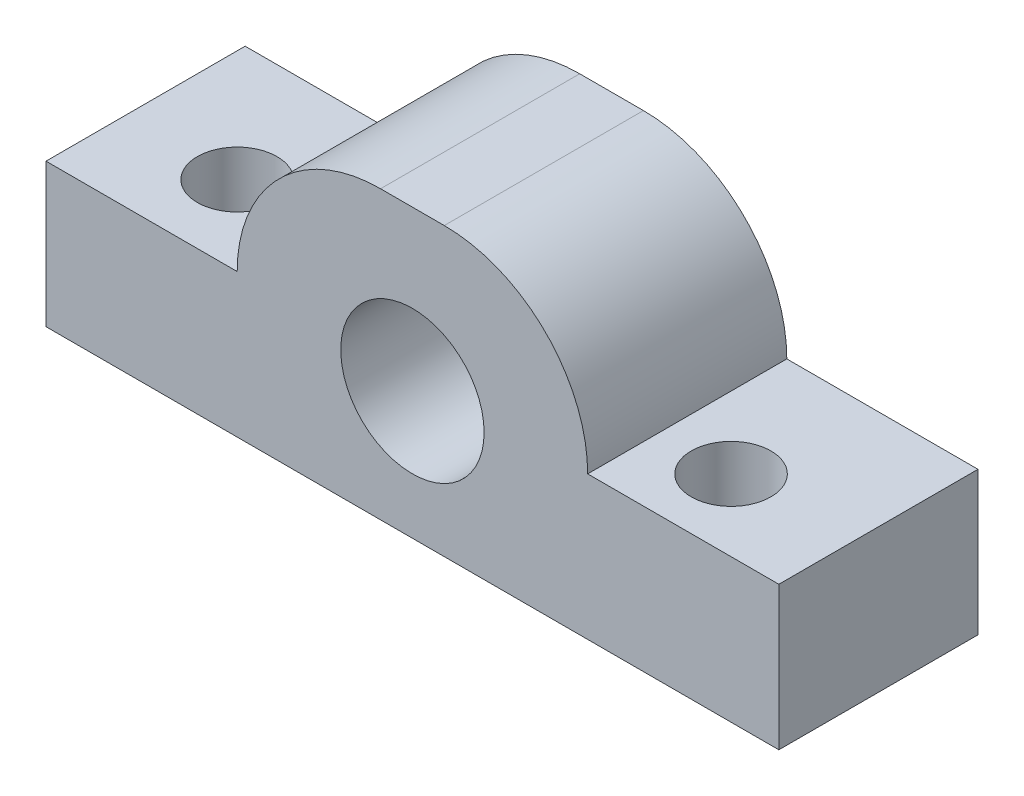
SolidWorks part; units mm, degrees
material "Plain Carbon Steel"
ref_plane "Front Plane" through (0, 0, 0) normal (0, 0, 1) x (1, 0, 0)
ref_plane "Top Plane" through (0, 0, 0) normal (0, 1, 0) x (1, 0, 0)
ref_plane "Right Plane" through (0, 0, 0) normal (1, 0, 0) x (0, 0, -1)
sketch "Pillow Block Profile" plane through (0, 0, 0) normal (0, 0, 1) x (1, 0, 0)
  line L0 (0, 0) -> (0, 29.5265) construction
  line L1 (46, 0) -> (-46, 0)
  line L2 (-46, 0) -> (-46, 18)
  line L3 (-46, 18) -> (-22, 18)
  line L4 (-4, 36) -> (4, 36)
  line L5 (46, 0) -> (46, 18)
  line L6 (46, 18) -> (22, 18)
  arc A0 (-22, 18) -> (-4, 36) centre (-4, 18) cw
  arc A1 (22, 18) -> (4, 36) centre (4, 18) ccw
  circle A2 centre (0, 16) radius 9
  point P14 (0, 36)
  dimension "D2" = 18
  dimension "D5" = 18
  dimension "D1" = 92
  dimension "D3" = 44
  dimension "D4" = 36
  dimension "D6" = 16
extrude "Pillow Block Body" add sketch "Pillow Block Profile" along normal mid plane 25
hole_wizard "Mounting Holes 2xØ10" positions "3DSketch1" profile "Sketch2" hole size "Ø10.0" standard "ISO" end condition up to next
sketch3d "3DSketch1"
  line L0 (-46, 18, 12.5) -> (-46, 18, -12.5) construction
  line L1 (-22, 18, 12.5) -> (-46, 18, 12.5) construction
  line L2 (46, 18, 12.5) -> (22, 18, 12.5) construction
  line L3 (46, 18, 12.5) -> (46, 18, -12.5) construction
  point P0 (-32, 18, 2.5)
  point P2 (31, 18, 3.5)
  dimension "D1" = 14
  dimension "D2" = 10
  dimension "D3" = 9
  dimension "D4" = 15
sketch "Sketch2" plane through (-32, 18, 2.5) normal (1, 0, 0) x (0, 0, 1)
  line L0 (0, 0) -> (0, 18)
  line L1 (0, 18) -> (5, 18)
  line L2 (5, 18) -> (5, 0)
  line L5 (5, 0) -> (0, 0)
  line L11 (0, -6.35) -> (0, 107.95) construction
  dimension "Thru Hole Dia." = 10
  dimension "Thru Hole Depth" = 18
